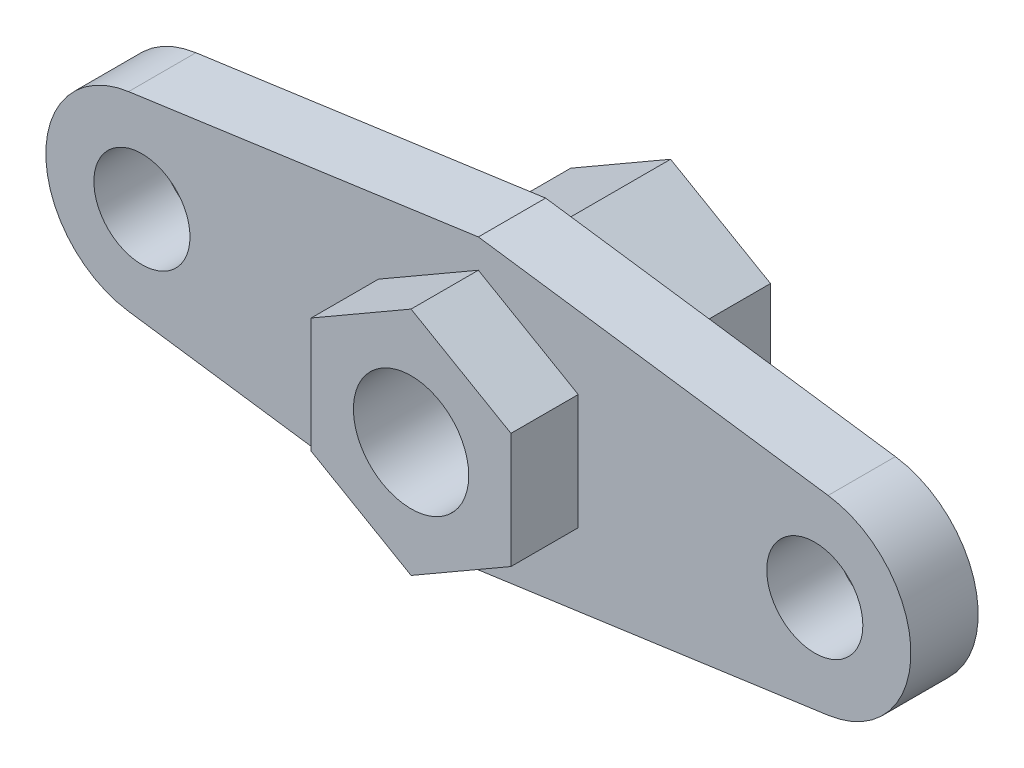
from build123d import *

# Parameters (mm, degrees)
LINK_PLATE_PROFILE_R  = 5
LINK_PLATE_DEPTH      = 3.5
FRONT_HEX_BOSS_DEPTH  = 10.5
REAR_HEX_BOSS_DEPTH   = 16.5
CENTRE_BORE_PROFILE_R = 6
CENTRE_BORE_12_DEPTH  = 72.572811156


with BuildPart() as part:
    # Link Plate Profile → Link Plate (new, symmetric)
    with BuildSketch(Plane.XY):
        with BuildLine():
            Line((55.952356647, 9.903324931), (19.565217391, 15))
            Line((19.565217391, 15), (-16.821921865, 9.903324931))
            ThreePointArc((-16.821921865, 9.903324931), (-25.434782609, 0), (-16.821921865, -9.903324931))
            Line((-16.821921865, -9.903324931), (19.565217391, -15))
            Line((19.565217391, -15), (55.952356647, -9.903324931))
            ThreePointArc((55.952356647, -9.903324931), (64.565217391, 0), (55.952356647, 9.903324931))
        make_face()
        with Locations((-15.434782609, 0)):
            Circle(LINK_PLATE_PROFILE_R, mode=Mode.SUBTRACT)
        Polygon((9.172912546, 6), (19.565217391, 12), (29.957522237, 6), (29.957522237, -6), (19.565217391, -12), (9.172912546, -6), align=None, mode=Mode.SUBTRACT)
        with Locations((54.565217391, 0)):
            Circle(LINK_PLATE_PROFILE_R, mode=Mode.SUBTRACT)
    extrude(amount=LINK_PLATE_DEPTH, both=True)

    # Front Hex Profile → Front Hex Boss (add)
    with BuildSketch(Plane.XY):
        Polygon((9.172912546, 6), (9.172912546, -6), (19.565217391, -12), (29.957522237, -6), (29.957522237, 6), (19.565217391, 12), align=None)
    extrude(amount=FRONT_HEX_BOSS_DEPTH)

    # Rear Hex Profile → Rear Hex Boss (add)
    with BuildSketch(Plane(origin=(0, 0, 0), x_dir=(-1, 0, 0), z_dir=(0, 0, -1))):
        Polygon((-9.172912546, 6), (-19.565217391, 12), (-29.957522237, 6), (-29.957522237, -6), (-19.565217391, -12), (-9.172912546, -6), align=None)
    extrude(amount=REAR_HEX_BOSS_DEPTH)

    # Centre Bore Profile → Centre Bore Ø12 (cut, through all)
    with BuildSketch(Plane.XY.offset(10.5)):
        with Locations((19.565217391, 0)):
            Circle(CENTRE_BORE_PROFILE_R)
    extrude(amount=-CENTRE_BORE_12_DEPTH, mode=Mode.SUBTRACT)


solid = part.part
